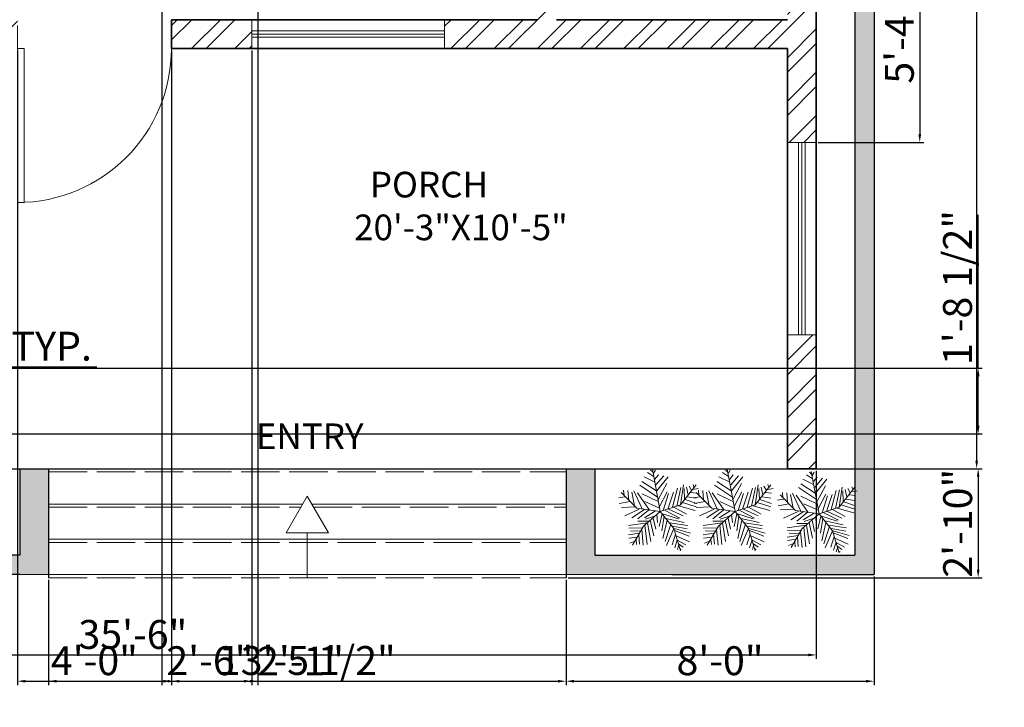
# Model space of a CAD drawing. Units: inches. Extents: x 418 to 1041, y 2094 to 2761.
# Tile 3 of 5: x 723 to 1030, y 2094 to 2308. Entities that reach past the tile are written whole.
import ezdxf

# ---------------------------------------------------------------- set-up
doc = ezdxf.new("R2010")
doc.units = ezdxf.units.IN
doc.linetypes.add('ACAD_ISO02W100', pattern=[15, 12, -3])
for name, color, linetype, lineweight in [('A-ANNO-DIMS', 2, 'Continuous', 18), ('A-ANNO-SYMB', 7, 'Continuous', 18), ('A-AREA-IDEN', 7, 'Continuous', 18), ('A-DOOR', 4, 'Continuous', 18), ('A-FLOR', 7, 'Continuous', 25), ('A-FLOR-STRS', 7, 'Continuous', 18), ('A-FLOR-STRS-HIDN', 8, 'ACAD_ISO02W100', 13), ('A-GLAZ', 244, 'Continuous', 18), ('A-WALL', 7, 'Continuous', 35), ('A-WALL-PATT', 252, 'Continuous', 13), ('L-PLNT', 3, 'Continuous', 13), ('L-WALL', 7, 'Continuous', 25), ('L-WALL-PATT', 252, 'Continuous', 13)]:
    doc.layers.add(name, color=color, linetype=linetype, lineweight=lineweight)
doc.styles.get("Standard").update_dxf_attribs({"font": 'arial.ttf'})
doc.dimstyles.new('ISO-25', dxfattribs={"dimtxt": 9, "dimasz": 2.5, "dimexe": 1.25, "dimexo": 0.625, "dimtad": 1, "dimlunit": 3, "dimtxsty": 'Standard', "dimcen": 2.5, "dimadec": 0, "dimazin": 0, "dimtfac": 1, "dimtmove": 0, "dimatfit": 3, "dimfxl": 1, "dimarcsym": 0})

# ---------------------------------------------------------------- blocks, each defined once
blk = doc.blocks.new('*U3')
for p, q in [((0, 0), (0, 6)), ((40, 0), (40, 6))]:
    blk.add_line(p, q)
blk.add_lwpolyline([(0, 0), (0, -40), (1.75, -40), (1.75, 0)], close=True)
blk.add_arc((0, 0), 40, 270, 0)
blk = doc.blocks.new('*U14')
for p, q in [((-10.186, 53.64), (-13.084, 55.962)), ((0, 0), (-10.5, 57)), ((-9.099, 51.782), (-6.563, 55.962)), ((-5.114, 28.097), (-24.676, 40.636)), ((-7.288, 39.707), (-21.778, 46.673)), ((-8.737, 47.138), (-17.069, 52.711)), ((-7.65, 43.423), (-2.578, 49.46)), ((-5.839, 35.992), (4.667, 48.067)), ((-5.114, 27.632), (10.463, 46.673)), ((-48.585, 21.131), (-49.309, 29.026)), ((-43.513, 28.561), (-42.427, 15.558)), ((-35.544, 28.097), (-24.314, 3.947)), ((-3.665, 19.273), (-27.574, 35.527)), ((-2.941, 16.486), (8.652, 37.85)), ((-1.129, 6.734), (9.014, 26.704)), ((16.259, 5.805), (23.142, 31.348)), ((22.055, 7.198), (27.489, 32.277)), ((27, 9), (48, 36)), ((27.127, 9.056), (31.112, 35.992)), ((31.836, 30.883), (32.561, 16.486)), ((35.096, 32.741), (37.27, 22.524)), ((38.719, 34.134), (41.979, 28.561)), ((43.791, 29.954), (51.036, 30.883)), ((44.153, 36.456), (45.239, 32.741)), ((-47.498, 19.737), (-55.83, 18.344)), ((-40.615, 13.7), (-55.105, 10.913)), ((-31.5, 4.5), (-52.5, 25.5)), ((-38.442, 26.239), (-34.819, 7.663)), ((-14.533, 2.09), (-30.834, 25.31)), ((-24.314, 23.917), (-2.941, 13.7)), ((-20.691, 13.7), (-1.129, 4.876)), ((3.942, 1.625), (11.187, 24.381)), ((10.101, 3.483), (17.708, 26.239)), ((33.285, 16.486), (48.862, 10.913)), ((36.183, 19.737), (48.137, 17.88)), ((40.53, 25.775), (48.862, 24.846)), ((-33.37, 6.269), (-52.207, 5.34)), ((-28.299, 3.483), (-47.86, -5.805)), ((-21.416, 3.018), (-38.079, -8.128)), ((0, 0), (-31.5, 4.5)), ((-15.982, 2.09), (-30.11, -9.521)), ((0, 0), (-22.5, -19.5)), ((-6.563, 1.161), (-21.416, -8.128)), ((0, 0), (27, 9)), ((0, 0), (18, -22.5)), ((6.478, 1.625), (26.04, -8.592)), ((11.187, 3.483), (30.749, -5.805)), ((18.07, 5.805), (35.096, -3.483)), ((24.229, 7.663), (46.688, 1.625)), ((29.662, 12.307), (48.137, 6.269)), ((-15.257, -12.772), (-30.11, -12.772)), ((-6.563, -5.805), (-19.967, -9.985)), ((-13.446, -11.378), (-8.737, -32.741)), ((-9.461, -8.592), (-6.201, -23.453)), ((-4.752, -3.483), (-3.665, -14.629)), ((2.493, -3.019), (-1.491, -20.202)), ((1.769, -2.555), (24.229, -9.521)), ((5.029, -6.27), (2.131, -25.775)), ((9.014, -11.378), (3.58, -35.992)), ((7.565, -9.056), (32.198, -14.629)), ((-17.431, -15.094), (-42.789, -18.809)), ((-24.314, -21.596), (-42.427, -22.06)), ((-26.849, -26.24), (-40.253, -25.775)), ((-22.5, -19.5), (-37.5, -45)), ((-25.038, -23.918), (-22.865, -45.281)), ((-20.691, -18.345), (-17.793, -44.352)), ((-17.069, -15.094), (-12.721, -40.172)), ((14.085, -16.951), (6.478, -40.172)), ((18.07, -22.524), (8.289, -45.745)), ((12.274, -15.094), (36.907, -18.809)), ((16.259, -19.738), (36.183, -22.989)), ((18, -22.5), (27, -52.5)), ((18.433, -22.524), (40.53, -29.026)), ((19.157, -25.311), (38.719, -33.206)), ((-28.299, -29.026), (-42.789, -31.348)), ((-30.834, -34.135), (-42.427, -35.528)), ((-32.646, -36.921), (-31.921, -44.352)), ((-29.023, -30.884), (-27.936, -43.887)), ((20.244, -30.419), (15.897, -44.816)), ((22.78, -37.85), (19.519, -48.532)), ((21.331, -32.741), (39.081, -40.636)), ((22.78, -38.314), (34.372, -44.816)), ((-34.457, -39.708), (-40.978, -42.494)), ((24.591, -45.745), (23.142, -50.854)), ((24.591, -43.423), (30.749, -47.603)), ((26.764, -49.925), (28.213, -50.854))]:
    blk.add_line(p, q)
blk = doc.blocks.new('*D16')
at = {"layer": 'A-ANNO-DIMS', "color": 0, "lineweight": -2, "transparency": 16777216}
for p, q in [((972.18, 2666.03), (1022.79, 2666.03)), ((1021.54, 2663.53), (1021.54, 2170.53)), ((972.18, 2168.03), (1022.79, 2168.03))]:
    blk.add_line(p, q, dxfattribs=at)
at = {"layer": 'A-ANNO-DIMS', "color": 0, "transparency": 16777216}
for points in [[(1021.13, 2663.53), (1021.96, 2663.53), (1021.54, 2666.03)], [(1021.13, 2170.53), (1021.96, 2170.53), (1021.54, 2168.03)]]:
    blk.add_solid(points, dxfattribs=at)
at = {"layer": 'Defpoints', "color": 0, "transparency": 16777216}
for p in [(971.56, 2666.03), (971.56, 2168.03), (1021.54, 2168.03)]:
    blk.add_point(p, dxfattribs=at)
at = {"layer": 'A-ANNO-DIMS', "color": 0, "transparency": 16777216, "insert": (1016.32, 2417.03), "char_height": 9, "attachment_point": 5, "rotation": 90}
blk.add_mtext('41\'-6"', dxfattribs=at)
blk = doc.blocks.new('*D17')
at = {"layer": 'A-ANNO-DIMS', "color": 0, "lineweight": -2, "transparency": 16777216}
for p, q in [((545.56, 2167.4), (545.56, 2108.72)), ((971.56, 2167.4), (971.56, 2108.72)), ((548.06, 2109.97), (969.06, 2109.97))]:
    blk.add_line(p, q, dxfattribs=at)
at = {"layer": 'A-ANNO-DIMS', "color": 0, "transparency": 16777216}
for points in [[(548.06, 2110.39), (548.06, 2109.55), (545.56, 2109.97)], [(969.06, 2110.39), (969.06, 2109.55), (971.56, 2109.97)]]:
    blk.add_solid(points, dxfattribs=at)
at = {"layer": 'Defpoints', "color": 0, "transparency": 16777216}
for p in [(545.56, 2168.03), (971.56, 2168.03), (971.56, 2109.97)]:
    blk.add_point(p, dxfattribs=at)
at = {"layer": 'A-ANNO-DIMS', "color": 0, "transparency": 16777216, "insert": (758.56, 2115.19), "char_height": 9, "attachment_point": 5}
blk.add_mtext('35\'-6"', dxfattribs=at)
blk = doc.blocks.new('WIN-60IN')
for p, q in [((0, 5.5), (60, 5.5)), ((0, 4.5), (60, 4.5)), ((0, 3.5), (60, 3.5))]:
    blk.add_line(p, q)
blk.add_lwpolyline([(0, 9), (60, 9), (60, 0), (0, 0)], close=True)
blk = doc.blocks.new('*D29')
at = {"layer": 'A-ANNO-DIMS', "color": 0, "lineweight": -2, "transparency": 16777216}
for p, q in [((645.38, 2200.08), (645.38, 2201.03)), ((647.54, 2200.08), (647.54, 2201.03)), ((642.88, 2199.78), (640.38, 2199.78)), ((645.38, 2199.78), (647.54, 2199.78)), ((650.04, 2199.78), (747.37, 2199.78))]:
    blk.add_line(p, q, dxfattribs=at)
at = {"layer": 'A-ANNO-DIMS', "color": 0, "transparency": 16777216}
for points in [[(642.88, 2200.2), (642.88, 2199.36), (645.38, 2199.78)], [(650.04, 2200.2), (650.04, 2199.36), (647.54, 2199.78)]]:
    blk.add_solid(points, dxfattribs=at)
at = {"layer": 'Defpoints', "color": 0, "transparency": 16777216}
for p in [(645.38, 2199.46), (647.54, 2199.78), (647.54, 2199.46)]:
    blk.add_point(p, dxfattribs=at)
at = {"layer": 'A-ANNO-DIMS', "color": 0, "transparency": 16777216, "insert": (699.96, 2205.06), "char_height": 9, "attachment_point": 5}
blk.add_mtext('KNOB 0\'-2" TYP.', dxfattribs=at)
blk = doc.blocks.new('*D50')
at = {"layer": 'A-ANNO-DIMS', "color": 0, "lineweight": -2, "transparency": 16777216}
for p, q in [((972.18, 2333.53), (1005.06, 2333.53)), ((1003.81, 2331.03), (1003.81, 2272.26)), ((972.18, 2269.76), (1005.06, 2269.76))]:
    blk.add_line(p, q, dxfattribs=at)
at = {"layer": 'A-ANNO-DIMS', "color": 0, "transparency": 16777216}
for points in [[(1003.39, 2331.03), (1004.22, 2331.03), (1003.81, 2333.53)], [(1003.39, 2272.26), (1004.22, 2272.26), (1003.81, 2269.76)]]:
    blk.add_solid(points, dxfattribs=at)
at = {"layer": 'Defpoints', "color": 0, "transparency": 16777216}
for p in [(971.56, 2333.53), (971.56, 2269.76), (1003.81, 2269.76)]:
    blk.add_point(p, dxfattribs=at)
at = {"layer": 'A-ANNO-DIMS', "color": 0, "transparency": 16777216, "insert": (998.61, 2301.64), "char_height": 9, "attachment_point": 5, "rotation": 90}
blk.add_mtext('5\'-4"', dxfattribs=at)
blk = doc.blocks.new('*D53')
at = {"layer": 'A-ANNO-DIMS', "color": 0, "lineweight": -2, "transparency": 16777216}
for p, q in [((770.56, 2298.4), (770.56, 2100.53)), ((795.65, 2298.4), (795.65, 2100.53)), ((773.06, 2101.78), (793.15, 2101.78)), ((795.65, 2101.78), (823.48, 2101.78))]:
    blk.add_line(p, q, dxfattribs=at)
at = {"layer": 'A-ANNO-DIMS', "color": 0, "transparency": 16777216}
for points in [[(773.06, 2102.19), (773.06, 2101.36), (770.56, 2101.78)], [(793.15, 2102.19), (793.15, 2101.36), (795.65, 2101.78)]]:
    blk.add_solid(points, dxfattribs=at)
at = {"layer": 'Defpoints', "color": 0, "transparency": 16777216}
for p in [(770.56, 2299.03), (795.65, 2299.03), (795.65, 2101.78)]:
    blk.add_point(p, dxfattribs=at)
at = {"layer": 'A-ANNO-DIMS', "color": 0, "transparency": 16777216, "insert": (810.82, 2106.92), "char_height": 9, "attachment_point": 5}
blk.add_mtext('2\'-1"', dxfattribs=at)
blk = doc.blocks.new('*D54')
at = {"layer": 'A-ANNO-DIMS', "color": 0, "lineweight": -2, "transparency": 16777216}
for p, q in [((732.29, 2133.4), (732.29, 2100.53)), ((893.56, 2133.4), (893.56, 2100.53)), ((734.79, 2101.78), (891.06, 2101.78))]:
    blk.add_line(p, q, dxfattribs=at)
at = {"layer": 'A-ANNO-DIMS', "color": 0, "transparency": 16777216}
for points in [[(734.79, 2102.19), (734.79, 2101.36), (732.29, 2101.78)], [(891.06, 2102.19), (891.06, 2101.36), (893.56, 2101.78)]]:
    blk.add_solid(points, dxfattribs=at)
at = {"layer": 'Defpoints', "color": 0, "transparency": 16777216}
for p in [(732.29, 2134.03), (893.56, 2134.03), (893.56, 2101.78)]:
    blk.add_point(p, dxfattribs=at)
at = {"layer": 'A-ANNO-DIMS', "color": 0, "transparency": 16777216, "insert": (812.92, 2107.06), "char_height": 9, "attachment_point": 5}
blk.add_mtext('13\'-5 1/2"', dxfattribs=at)
blk = doc.blocks.new('*D55')
at = {"layer": 'A-ANNO-DIMS', "color": 0, "lineweight": -2, "transparency": 16777216}
for p, q in [((893.56, 2133.4), (893.56, 2100.53)), ((989.56, 2134.4), (989.56, 2100.53)), ((896.06, 2101.78), (987.06, 2101.78))]:
    blk.add_line(p, q, dxfattribs=at)
at = {"layer": 'A-ANNO-DIMS', "color": 0, "transparency": 16777216}
for points in [[(896.06, 2102.19), (896.06, 2101.36), (893.56, 2101.78)], [(987.06, 2102.19), (987.06, 2101.36), (989.56, 2101.78)]]:
    blk.add_solid(points, dxfattribs=at)
at = {"layer": 'Defpoints', "color": 0, "transparency": 16777216}
for p in [(893.56, 2134.03), (989.56, 2135.03), (989.56, 2101.78)]:
    blk.add_point(p, dxfattribs=at)
at = {"layer": 'A-ANNO-DIMS', "color": 0, "transparency": 16777216, "insert": (941.56, 2107), "char_height": 9, "attachment_point": 5}
blk.add_mtext('8\'-0"', dxfattribs=at)
blk = doc.blocks.new('*D56')
at = {"layer": 'A-ANNO-DIMS', "color": 0, "lineweight": -2, "transparency": 16777216}
for p, q in [((894.18, 2168.03), (1023.26, 2168.03)), ((1022.01, 2165.53), (1022.01, 2136.53)), ((894.18, 2134.03), (1023.26, 2134.03))]:
    blk.add_line(p, q, dxfattribs=at)
at = {"layer": 'A-ANNO-DIMS', "color": 0, "transparency": 16777216}
for points in [[(1021.6, 2165.53), (1022.43, 2165.53), (1022.01, 2168.03)], [(1021.6, 2136.53), (1022.43, 2136.53), (1022.01, 2134.03)]]:
    blk.add_solid(points, dxfattribs=at)
at = {"layer": 'Defpoints', "color": 0, "transparency": 16777216}
for p in [(893.56, 2168.03), (893.56, 2134.03), (1022.01, 2134.03)]:
    blk.add_point(p, dxfattribs=at)
at = {"layer": 'A-ANNO-DIMS', "color": 0, "transparency": 16777216, "insert": (1016.79, 2151.03), "char_height": 9, "attachment_point": 5, "rotation": 90}
blk.add_mtext('2\'-10"', dxfattribs=at)
blk = doc.blocks.new('*D57')
at = {"layer": 'A-ANNO-DIMS', "color": 0, "lineweight": -2, "transparency": 16777216}
for p, q in [((722.56, 2298.4), (722.56, 2100.53)), ((770.56, 2298.4), (770.56, 2100.53)), ((725.06, 2101.78), (768.06, 2101.78))]:
    blk.add_line(p, q, dxfattribs=at)
at = {"layer": 'A-ANNO-DIMS', "color": 0, "transparency": 16777216}
for points in [[(725.06, 2102.19), (725.06, 2101.36), (722.56, 2101.78)], [(768.06, 2102.19), (768.06, 2101.36), (770.56, 2101.78)]]:
    blk.add_solid(points, dxfattribs=at)
at = {"layer": 'Defpoints', "color": 0, "transparency": 16777216}
for p in [(722.56, 2299.03), (770.56, 2299.03), (770.56, 2101.78)]:
    blk.add_point(p, dxfattribs=at)
at = {"layer": 'A-ANNO-DIMS', "color": 0, "transparency": 16777216, "insert": (746.56, 2107), "char_height": 9, "attachment_point": 5}
blk.add_mtext('4\'-0"', dxfattribs=at)
blk = doc.blocks.new('*D59')
at = {"layer": 'A-ANNO-DIMS', "color": 0, "lineweight": -2, "transparency": 16777216}
for p, q in [((767.56, 2582.4), (767.56, 2100.53)), ((797.56, 2582.4), (797.56, 2100.53)), ((770.06, 2101.78), (795.06, 2101.78))]:
    blk.add_line(p, q, dxfattribs=at)
at = {"layer": 'A-ANNO-DIMS', "color": 0, "transparency": 16777216}
for points in [[(770.06, 2102.19), (770.06, 2101.36), (767.56, 2101.78)], [(795.06, 2102.19), (795.06, 2101.36), (797.56, 2101.78)]]:
    blk.add_solid(points, dxfattribs=at)
at = {"layer": 'Defpoints', "color": 0, "transparency": 16777216}
for p in [(767.56, 2583.03), (797.56, 2583.03), (797.56, 2101.78)]:
    blk.add_point(p, dxfattribs=at)
at = {"layer": 'A-ANNO-DIMS', "color": 0, "transparency": 16777216, "insert": (782.56, 2107), "char_height": 9, "attachment_point": 5}
blk.add_mtext('2\'-6"', dxfattribs=at)
blk = doc.blocks.new('*D69')
at = {"layer": 'A-ANNO-DIMS', "color": 0, "lineweight": -2, "transparency": 16777216}
for p, q in [((1022.01, 2199.37), (1022.01, 2247.17)), ((656.98, 2199.37), (1023.26, 2199.37)), ((1022.01, 2181.4), (1022.01, 2196.87)), ((656.98, 2178.9), (1023.26, 2178.9))]:
    blk.add_line(p, q, dxfattribs=at)
at = {"layer": 'A-ANNO-DIMS', "color": 0, "transparency": 16777216}
for points in [[(1021.6, 2196.87), (1022.43, 2196.87), (1022.01, 2199.37)], [(1021.6, 2181.4), (1022.43, 2181.4), (1022.01, 2178.9)]]:
    blk.add_solid(points, dxfattribs=at)
at = {"layer": 'Defpoints', "color": 0, "transparency": 16777216}
for p in [(656.36, 2199.37), (1022.01, 2199.37), (656.36, 2178.9)]:
    blk.add_point(p, dxfattribs=at)
at = {"layer": 'A-ANNO-DIMS', "color": 0, "transparency": 16777216, "insert": (1016.74, 2224.52), "char_height": 9, "attachment_point": 5, "rotation": 90}
blk.add_mtext('1\'-8 1/2"', dxfattribs=at)

msp = doc.modelspace()

# ---------------------------------------------------------------- hatches: boundary and pattern name
at = {"layer": 'A-WALL-PATT'}
h = msp.add_hatch(dxfattribs=at)
h.set_pattern_fill('ANSI32', color=256)
h.paths.add_polyline_path([(671.558, 2308.025), (554.558, 2308.025), (554.558, 2366.352), (545.558, 2366.352), (545.558, 2168.025), (555.667, 2168.025), (555.667, 2177.025), (554.558, 2177.025), (554.558, 2302.025), (671.558, 2302.025)])
h.paths.add_polyline_path([(719.558, 2299.025), (722.558, 2299.025), (722.558, 2306.225), (722.558, 2308.025), (707.558, 2308.025), (707.558, 2302.025), (710.558, 2302.025), (710.558, 2177.025), (665.344, 2177.025), (665.344, 2168.025), (719.558, 2168.025)])
h.paths.add_polyline_path([(605.344, 2177.025), (576.667, 2177.025), (576.667, 2168.025), (605.344, 2168.025)], flags=17)
h.paths.add_polyline_path([(795.654, 2308.025), (770.558, 2308.025), (770.558, 2299.025), (795.654, 2299.025)])
h.paths.add_polyline_path([(971.558, 2333.525), (962.558, 2333.525), (962.558, 2308.025), (890.558, 2308.025), (890.558, 2311.025), (886.058, 2311.025), (884.558, 2311.025), (884.558, 2308.025), (855.654, 2308.025), (855.654, 2299.025), (962.558, 2299.025), (962.558, 2269.763), (971.558, 2269.763)])
h.paths.add_polyline_path([(971.558, 2209.763), (962.558, 2209.763), (962.558, 2168.025), (971.558, 2168.025)])
h.paths.add_polyline_path([(971.558, 2422.525), (962.558, 2422.525), (962.558, 2386.025), (845.558, 2386.025), (845.558, 2380.025), (884.558, 2380.025), (884.558, 2341.025), (890.558, 2341.025), (890.558, 2380.025), (962.558, 2380.025), (962.558, 2354.525), (971.558, 2354.525)])
h.paths.add_polyline_path([(716.558, 2471.025), (651.558, 2471.025), (651.558, 2474.025), (647.058, 2474.025), (645.558, 2474.025), (645.558, 2471.025), (554.558, 2471.025), (554.558, 2484.525), (545.558, 2484.525), (545.558, 2426.352), (554.558, 2426.352), (554.558, 2465.025), (716.558, 2465.025)])
h.paths.add_polyline_path([(554.558, 2561.611), (545.558, 2561.611), (545.558, 2505.525), (554.558, 2505.525), (554.558, 2519.025), (645.558, 2519.025), (645.558, 2504.025), (651.558, 2504.025), (651.558, 2519.025), (716.558, 2519.025), (716.558, 2528.025), (710.558, 2528.025), (710.558, 2525.025), (554.558, 2525.025)])
h.paths.add_polyline_path([(971.558, 2561.025), (962.558, 2561.025), (962.558, 2525.025), (806.558, 2525.025), (806.558, 2528.025), (800.558, 2528.025), (800.558, 2380.025), (809.558, 2380.025), (809.558, 2386.025), (806.558, 2386.025), (806.558, 2519.025), (962.558, 2519.025), (962.558, 2482.525), (971.558, 2482.525)])
h.paths.add_polyline_path([(854.558, 2666.025), (769.058, 2666.025), (769.058, 2657.025), (800.558, 2657.025), (800.558, 2589.025), (797.558, 2589.025), (797.558, 2583.025), (800.558, 2583.025), (800.558, 2564.025), (806.558, 2564.025), (806.558, 2657.025), (854.558, 2657.025)])
h.paths.add_polyline_path([(971.558, 2666.025), (914.558, 2666.025), (914.558, 2657.025), (962.558, 2657.025), (962.558, 2621.025), (971.558, 2621.025)])
h.paths.add_polyline_path([(748.058, 2666.025), (662.558, 2666.025), (662.558, 2657.025), (710.558, 2657.025), (710.558, 2564.025), (716.558, 2564.025), (716.558, 2583.025), (767.558, 2583.025), (767.558, 2589.025), (716.558, 2589.025), (716.558, 2657.025), (748.058, 2657.025)])
h.paths.add_polyline_path([(602.558, 2666.025), (545.558, 2666.025), (545.558, 2621.611), (554.558, 2621.611), (554.558, 2657.025), (602.558, 2657.025)])
at = {"layer": 'L-WALL-PATT'}
h = msp.add_hatch(color=256, dxfattribs=at)
h.dxf.hatch_style = 1
h.paths.add_polyline_path([(533.558, 2678.025), (983.558, 2678.025), (983.558, 2141.025), (902.558, 2141.025), (902.558, 2168.025), (893.558, 2168.025), (893.558, 2135.025), (926.558, 2135.025), (989.558, 2135.025), (989.558, 2684.025), (527.558, 2684.025), (527.558, 2135.025), (723.29, 2135.025), (732.29, 2135.025), (732.29, 2168.025), (723.29, 2168.025), (723.29, 2141.025), (533.558, 2141.025)])

# ---------------------------------------------------------------- linework, layer by layer
at = {"layer": 'A-ANNO-SYMB'}
msp.add_line((812.924, 2134.025), (812.924, 2148.015), dxfattribs=at)
msp.add_lwpolyline([(812.924, 2159.461), (806.316, 2148.015), (819.532, 2148.015)], close=True, dxfattribs=at)
at = {"layer": 'A-FLOR'}
msp.add_line((719.558, 2168.025), (962.558, 2168.025), dxfattribs=at)
at = {"layer": 'A-FLOR-STRS'}
for p, q in [((732.29, 2157.025), (811.518, 2157.025)), ((814.33, 2157.025), (893.558, 2157.025)), ((732.29, 2146.025), (893.558, 2146.025)), ((723.29, 2135.025), (926.558, 2135.025))]:
    msp.add_line(p, q, dxfattribs=at)
at = {"layer": 'A-FLOR-STRS-HIDN'}
for p, q in [((732.29, 2167.025), (893.558, 2167.025)), ((732.29, 2156.025), (810.94, 2156.025)), ((814.907, 2156.025), (893.558, 2156.025)), ((732.29, 2145.025), (893.558, 2145.025)), ((732.29, 2134.025), (893.558, 2134.025))]:
    msp.add_line(p, q, dxfattribs=at)
at = {"layer": 'A-WALL'}
for p, q in [((971.558, 2666.025), (971.558, 2168.025)), ((770.558, 2299.025), (770.558, 2308.025)), ((770.558, 2308.025), (884.558, 2308.025)), ((890.558, 2308.025), (962.558, 2308.025)), ((770.558, 2299.025), (962.558, 2299.025)), ((962.558, 2299.025), (962.558, 2168.025)), ((962.558, 2168.025), (971.558, 2168.025))]:
    msp.add_line(p, q, dxfattribs=at)
at = {"layer": 'L-WALL'}
for p, q in [((989.558, 2684.025), (989.558, 2135.025)), ((983.558, 2678.025), (983.558, 2141.025)), ((723.29, 2168.025), (723.29, 2141.025)), ((732.29, 2168.025), (732.29, 2134.025)), ((893.558, 2168.025), (893.558, 2134.025)), ((902.558, 2168.025), (902.558, 2141.025)), ((723.29, 2141.025), (533.558, 2141.025)), ((902.558, 2141.025), (983.558, 2141.025)), ((723.29, 2135.025), (527.558, 2135.025)), ((926.558, 2135.025), (989.558, 2135.025))]:
    msp.add_line(p, q, dxfattribs=at)

# ---------------------------------------------------------------- block references
at = {"layer": 'A-DOOR', "xscale": 1.199999999999997, "yscale": 1.199999999999997, "zscale": 1.199999999999997}
msp.add_blockref('*U3', (722.558, 2299.025), dxfattribs=at)
at = {"layer": 'A-GLAZ'}
msp.add_blockref('WIN-60IN', (795.654, 2299.025), dxfattribs=at)
at = {"layer": 'A-GLAZ', "rotation": 270.0000000000002}
msp.add_blockref('WIN-60IN', (962.558, 2269.763), dxfattribs=at)
at = {"layer": 'L-PLNT', "xscale": 0.2319011365265418, "yscale": 0.2319011365265418, "zscale": 0.2319011365265418}
for p in [(922.951, 2154.646), (946.262, 2154.646), (972.427, 2153.926)]:
    msp.add_blockref('*U14', p, dxfattribs=at)

# ---------------------------------------------------------------- texts
at = {"layer": 'A-AREA-IDEN', "char_height": 8, "attachment_point": 1}
for s, width, insert in [('  PORCH\\P20\'-3"X10\'-5"', 63.10181, (827.519, 2260.605)), ('ENTRY', 35.84845, (796.877, 2182.131))]:
    msp.add_mtext_dynamic_manual_height_columns(s, width=width, gutter_width=12.5, heights=[0], dxfattribs=dict(at, insert=insert))

# ---------------------------------------------------------------- dimensions: what is measured, and where the dimension line sits
at = {"layer": 'A-ANNO-DIMS'}
for base, p1, p2, angle, override, picture, middle in [((1021.545, 2168.025), (971.558, 2666.025), (971.558, 2168.025), 90, {"dimclrd": 0, "dimclre": 0, "dimclrt": 0}, '*D16', (1016.325, 2417.025)), ((1003.808, 2269.763), (971.558, 2333.525), (971.558, 2269.763), 270, {"dimdec": 1, "dimlfac": 1, "dimrnd": 0, "dimzin": 1, "dimdsep": 46, "dimlunit": 4, "dimfrac": 2}, '*D50', (998.606, 2301.644)), ((1022.015, 2199.375), (656.359, 2178.9), (656.359, 2199.375), 90, {"dimdec": 1, "dimlfac": 1, "dimrnd": 0, "dimzin": 1, "dimdsep": 46, "dimlunit": 4, "dimfrac": 2}, '*D69', (1016.736, 2224.524)), ((1022.015, 2134.025), (893.558, 2168.025), (893.558, 2134.025), 90, {"dimdec": 1, "dimlfac": 1, "dimrnd": 0, "dimzin": 1, "dimdsep": 46, "dimlunit": 4, "dimfrac": 2}, '*D56', (1016.795, 2151.025))]:
    dim = msp.add_linear_dim(base=base, p1=p1, p2=p2, angle=angle, dimstyle='ISO-25', override=override, dxfattribs=at)
    dim.commit()
    dim.dimension.update_dxf_attribs({"geometry": picture, "text_midpoint": middle})
for base, p1, p2, override, picture, middle in [((797.558, 2101.775), (767.558, 2583.025), (797.558, 2583.025), {"dimdec": 1, "dimlfac": 1, "dimrnd": 0, "dimzin": 1, "dimdsep": 46, "dimlunit": 4, "dimfrac": 2}, '*D59', (782.558, 2106.996)), ((770.558, 2101.775), (722.558, 2299.025), (770.558, 2299.025), {"dimdec": 1, "dimlfac": 1, "dimrnd": 0, "dimzin": 1, "dimdsep": 46, "dimlunit": 4, "dimfrac": 2}, '*D57', (746.558, 2106.996)), ((795.654, 2101.775), (770.558, 2299.025), (795.654, 2299.025), {"dimdec": 1, "dimlfac": 1, "dimrnd": 0, "dimzin": 1, "dimdsep": 46, "dimlunit": 4, "dimfrac": 2}, '*D53', (810.818, 2106.919)), ((971.558, 2109.971), (545.558, 2168.025), (971.558, 2168.025), {"dimclrd": 0, "dimclre": 0, "dimclrt": 0}, '*D17', (758.558, 2115.194)), ((893.558, 2101.775), (732.29, 2134.025), (893.558, 2134.025), {"dimdec": 1, "dimlfac": 1, "dimrnd": 0, "dimzin": 1, "dimdsep": 46, "dimlunit": 4, "dimfrac": 2}, '*D54', (812.924, 2107.057)), ((989.558, 2101.775), (893.558, 2134.025), (989.558, 2135.025), {"dimdec": 1, "dimlfac": 1, "dimrnd": 0, "dimzin": 1, "dimdsep": 46, "dimlunit": 4, "dimfrac": 2}, '*D55', (941.558, 2106.996))]:
    dim = msp.add_linear_dim(base=base, p1=p1, p2=p2, dimstyle='ISO-25', override=override, dxfattribs=at)
    dim.commit()
    dim.dimension.update_dxf_attribs({"geometry": picture, "text_midpoint": middle})
dim = msp.add_linear_dim(base=(647.539, 2199.78), p1=(645.377, 2199.456), p2=(647.539, 2199.456), text='KNOB <> TYP.', dimstyle='ISO-25', override={"dimdec": 1, "dimlfac": 1, "dimrnd": 0, "dimzin": 1, "dimdsep": 46, "dimlunit": 4, "dimfrac": 2}, dxfattribs=at)
dim.commit()
dim.dimension.update_dxf_attribs({"geometry": '*D29', "text_midpoint": (699.956, 2205.062)})

doc.saveas('drawing.dxf')
